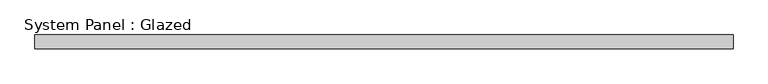
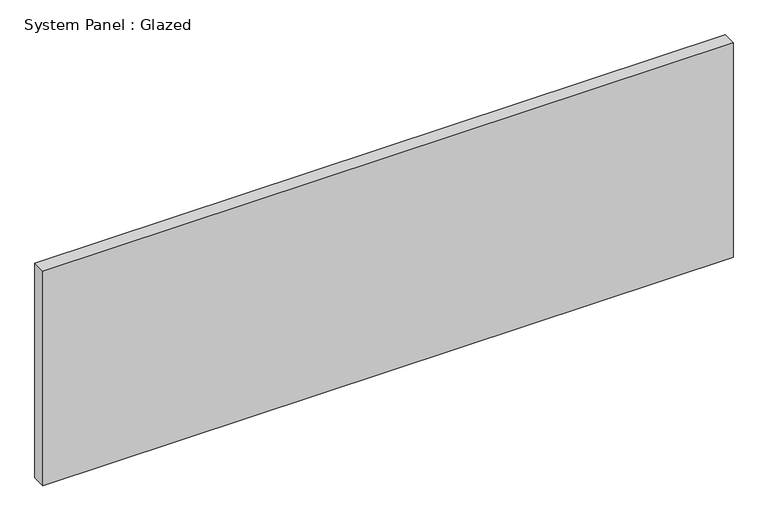
"""IFC4 building model written with IfcOpenShell, lengths in millimetres: plate geometry, System Panel : Glazed."""

from ifc_helpers import new_model, si_unit, origin, origin_with_axes, place, context, project, spatial, polyline, outline, extrude, source, transform, mapped, element, save


def system_panel_glazed_a0664fa1(model_context):
    return source(origin(), model_context, "Body", "SweptSolid", [
        extrude(outline(polyline([(638.1750001, 19.05), (-638.1750001, 19.05), (-638.1750001, 44.45), (638.1750001, 44.45), (638.1750001, 19.05)])), origin_with_axes(), (0.0, 0.0, 1.0), 419.1),
    ])


if __name__ == "__main__":
    model = new_model("IFC4")
    model_context = context("Model", 3, world=origin())
    ifc_project = project(units=[si_unit("LENGTHUNIT", "METRE", prefix="MILLI")], contexts=[model_context])
    site = spatial("IfcSite", under=ifc_project)
    building = spatial("IfcBuilding", under=site)
    placement = place(None, origin())
    system_panel_glazed_shape = system_panel_glazed_a0664fa1(model_context)
    element("IfcPlate", 1, ObjectType="System Panel : Glazed", at=placement, inside=building, context=model_context, shape_type="MappedRepresentation", body=[
        mapped(system_panel_glazed_shape, transform((0.0, 0.0, 0.0), x_axis=(1.0, 0.0, 0.0), y_axis=(0.0, 1.0, 0.0), z_axis=(0.0, 0.0, 1.0))),
    ])
    save(model, "model.ifc")

# Revit data of these elements
# Type "System Panel : Glazed"
#   Construction Type Id = "GSP4R"
#   Analytic Construction = "1/8 in Pilkington single glazing"
#   Visual Light Transmittance = 0.9
#   Solar Heat Gain Coefficient = 0.86
#   Heat Transfer Coefficient (U) = 1.18115 BTU/(h·ft²·°F)
#   Define Thermal Properties by = 1
# Element 1 (IfcPlate, "System Panel : Glazed")
#   Materials on its faces: "glass panel 223"
# Materials
#   "glass panel 223": class "Generic", colour RGB 120 120 120, transparency 0, Cost = 0
